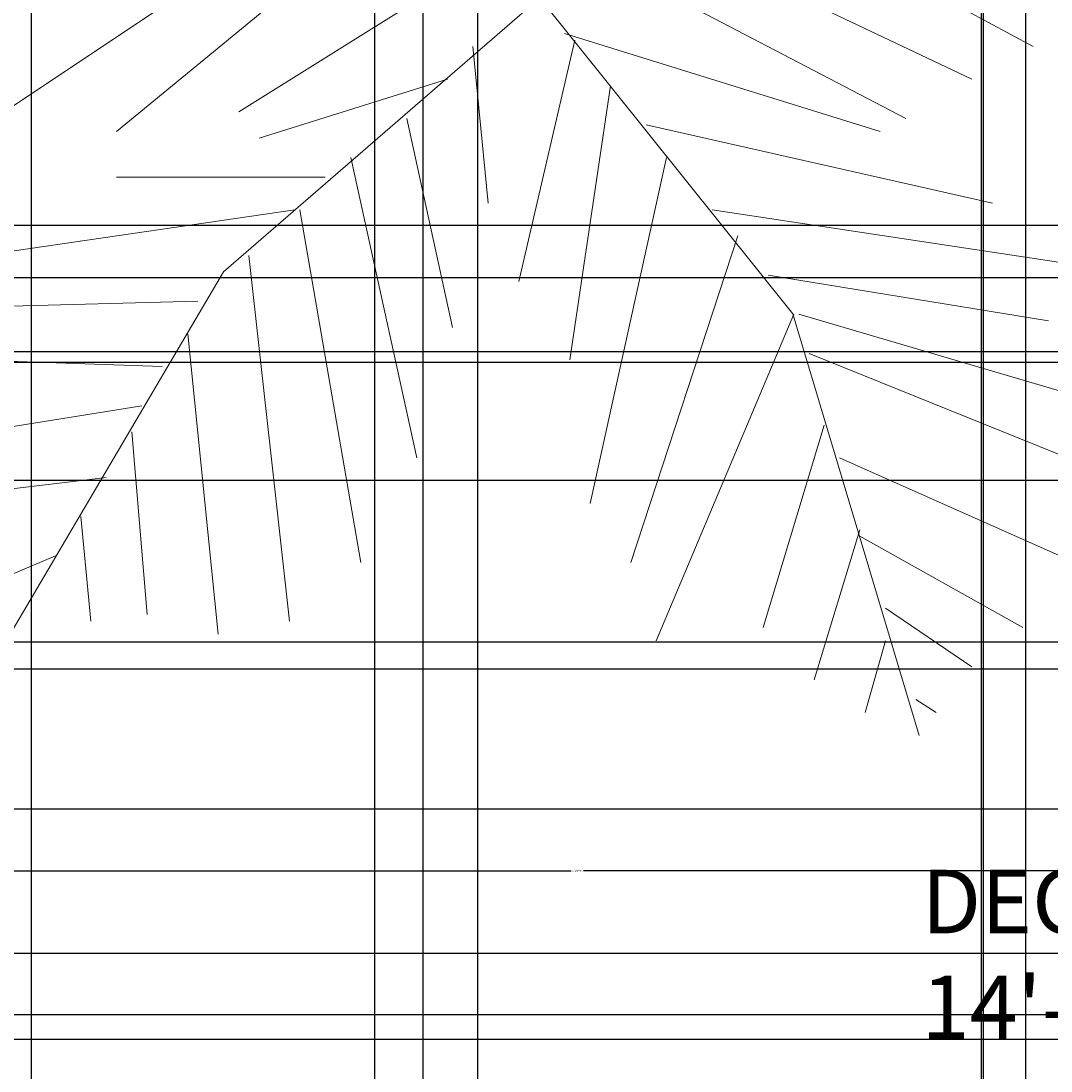
# Model space of a CAD drawing. Units: inches. Extents: x 818 to 1898, y 976 to 2364.
# Tile 62 of 96: x 1083 to 1180, y 1873 to 1972. Entities that reach past the tile are written whole.
import ezdxf

# ---------------------------------------------------------------- set-up
doc = ezdxf.new("R2010")
doc.units = ezdxf.units.IN
doc.header["$LTSCALE"] = 5
doc.header["$MEASUREMENT"] = 0
for name, color, linetype, lineweight in [('A-ANNO-DIMS', 2, 'Continuous', 18), ('A-AREA-IDEN', 7, 'Continuous', 18), ('L-PLNT-BEDS', 94, 'Continuous', 18)]:
    doc.layers.add(name, color=color, linetype=linetype, lineweight=lineweight)
doc.layers.add('L-PLNT', color=116, linetype='Continuous', lineweight=13, true_color=0x136734)
doc.styles.get("Standard").update_dxf_attribs({"font": 'arial.ttf'})
doc.dimstyles.get("Standard").update_dxf_attribs({"dimtxt": 0.18, "dimasz": 0.18, "dimexe": 0.18, "dimexo": 0.0625, "dimgap": 0.09, "dimtad": 0, "dimtih": 1, "dimtoh": 1, "dimdec": 4, "dimzin": 0, "dimdsep": 46, "dimtxsty": 'Standard', "dimcen": 0.09, "dimadec": 0, "dimazin": 0, "dimtfac": 1, "dimtdec": 4, "dimtofl": 0, "dimtmove": 0, "dimatfit": 3, "dimfxl": 1, "dimtolj": 1, "dimtzin": 0, "dimarcsym": 0})

# ---------------------------------------------------------------- blocks, each defined once
blk = doc.blocks.new('PALM-DECK')
for p, q in [((98.208, 77.483), (120.834, 65.14)), ((45.734, 73.779), (23.59, 58.967)), ((89.061, 74.397), (115.057, 62.054)), ((52.955, 72.546), (34.18, 57.116)), ((82.803, 71.928), (108.799, 58.35)), ((65.472, 71.311), (45.734, 58.967)), ((74.194, 69.769), (44.293, 43.854)), ((74.194, 69.769), (98.115, 39.868)), ((77.507, 65.757), (72.213, 42.922)), ((76.545, 66.373), (106.393, 57.116)), ((67.879, 65.14), (69.324, 50.328)), ((65.472, 62.054), (47.659, 56.499)), ((80.877, 61.436), (77.026, 35.515)), ((61.621, 58.35), (65.953, 38.601)), ((84.247, 57.734), (116.983, 50.328)), ((56.325, 54.648), (62.583, 26.258)), ((86.173, 54.648), (78.952, 21.938)), ((53.919, 52.795), (34.18, 52.795)), ((51.03, 49.71), (17.331, 44.773)), ((51.511, 49.71), (57.289, 16.383)), ((90.505, 49.71), (123.241, 44.773)), ((92.912, 47.242), (82.803, 16.383)), ((46.697, 45.389), (50.548, 10.828)), ((44.293, 43.854), (24.359, 9.967)), ((95.801, 43.538), (122.279, 39.218)), ((41.883, 41.069), (17.812, 40.452)), ((98.208, 39.836), (85.21, 8.977)), ((98.115, 39.868), (110.075, 0)), ((98.69, 39.836), (128.056, 31.195)), ((40.92, 37.983), (43.808, 9.593)), ((99.652, 36.132), (125.649, 25.64)), ((38.514, 34.897), (20.701, 35.515)), ((36.587, 31.195), (17.331, 28.109)), ((101.097, 29.344), (95.32, 10.211)), ((35.625, 28.726), (37.069, 11.446)), ((102.541, 26.258), (126.13, 15.766)), ((33.218, 24.406), (17.812, 22.554)), ((30.81, 20.703), (31.773, 10.828)), ((104.467, 19.469), (100.133, 5.273)), ((104.467, 18.852), (119.872, 10.211)), ((28.403, 16.999), (19.737, 13.297)), ((106.874, 12.063), (115.057, 6.508)), ((106.874, 8.977), (104.948, 2.187)), ((109.762, 3.422), (111.687, 2.187))]:
    blk.add_line(p, q)
blk = doc.blocks.new('*D29')
at = {"layer": 'A-ANNO-DIMS', "color": 0, "lineweight": -2, "ltscale": 5, "transparency": 16777216}
for p, q in [((1064.31, 1870.244), (1064.31, 1892.189)), ((1064.49, 1892.009), (1134.729, 1892.009)), ((1206.147, 1892.009), (1135.908, 1892.009)), ((1206.327, 1870.244), (1206.327, 1892.189))]:
    blk.add_line(p, q, dxfattribs=at)
at = {"layer": 'A-ANNO-DIMS', "color": 0, "ltscale": 5, "transparency": 16777216}
for points in [[(1064.49, 1892.039), (1064.49, 1891.979), (1064.31, 1892.009)], [(1206.147, 1892.039), (1206.147, 1891.979), (1206.327, 1892.009)]]:
    blk.add_solid(points, dxfattribs=at)
at = {"layer": 'Defpoints', "color": 0, "ltscale": 5, "transparency": 16777216}
for p in [(1206.327, 1892.009), (1064.31, 1870.181), (1206.327, 1870.181)]:
    blk.add_point(p, dxfattribs=at)
at = {"layer": 'A-ANNO-DIMS', "color": 0, "ltscale": 5, "transparency": 16777216, "insert": (1135.319, 1892.009), "char_height": 0.18, "attachment_point": 5}
blk.add_mtext('\\A1;142 TYP.', dxfattribs=at)
blk = doc.blocks.new('*D59')
at = {"layer": 'A-ANNO-DIMS', "color": 0, "lineweight": -2, "ltscale": 5, "transparency": 16777216}
for p, q in [((1251.643, 2300.393), (818.026, 2300.393)), ((818.206, 2300.213), (818.206, 1669.95)), ((818.206, 1039.323), (818.206, 1669.586)), ((896.051, 1039.143), (818.026, 1039.143))]:
    blk.add_line(p, q, dxfattribs=at)
at = {"layer": 'A-ANNO-DIMS', "color": 0, "ltscale": 5, "transparency": 16777216}
for points in [[(818.176, 2300.213), (818.236, 2300.213), (818.206, 2300.393)], [(818.176, 1039.323), (818.236, 1039.323), (818.206, 1039.143)]]:
    blk.add_solid(points, dxfattribs=at)
at = {"layer": 'Defpoints', "color": 0, "ltscale": 5, "transparency": 16777216}
for p in [(818.206, 2300.393), (1251.706, 2300.393), (896.114, 1039.143)]:
    blk.add_point(p, dxfattribs=at)
at = {"layer": 'A-ANNO-DIMS', "color": 0, "ltscale": 5, "transparency": 16777216, "insert": (818.206, 1669.768), "char_height": 0.18, "attachment_point": 5}
blk.add_mtext('\\A1;1261.2', dxfattribs=at)
blk = doc.blocks.new('*D61')
at = {"layer": 'A-ANNO-DIMS', "color": 0, "lineweight": -2, "ltscale": 5, "transparency": 16777216}
for p, q in [((1071.725, 1203.027), (1071.725, 2363.873)), ((1430.725, 1203.027), (1430.725, 2363.873)), ((1071.905, 2363.693), (1250.936, 2363.693)), ((1430.545, 2363.693), (1251.514, 2363.693))]:
    blk.add_line(p, q, dxfattribs=at)
at = {"layer": 'A-ANNO-DIMS', "color": 0, "ltscale": 5, "transparency": 16777216}
for points in [[(1071.905, 2363.723), (1071.905, 2363.663), (1071.725, 2363.693)], [(1430.545, 2363.723), (1430.545, 2363.663), (1430.725, 2363.693)]]:
    blk.add_solid(points, dxfattribs=at)
at = {"layer": 'Defpoints', "color": 0, "ltscale": 5, "transparency": 16777216}
for p in [(1430.725, 2363.693), (1071.725, 1202.964), (1430.725, 1202.964)]:
    blk.add_point(p, dxfattribs=at)
at = {"layer": 'A-ANNO-DIMS', "color": 0, "ltscale": 5, "transparency": 16777216, "insert": (1251.225, 2363.693), "char_height": 0.18, "attachment_point": 5}
blk.add_mtext('\\A1;359', dxfattribs=at)
blk = doc.blocks.new('*D74')
at = {"layer": 'A-ANNO-DIMS', "color": 0, "lineweight": -2, "ltscale": 5, "transparency": 16777216}
for p, q in [((1590.663, 1940.078), (818.026, 1940.078)), ((818.206, 1939.898), (818.206, 1925.76)), ((818.206, 1911.258), (818.206, 1925.396)), ((1590.663, 1911.078), (818.026, 1911.078))]:
    blk.add_line(p, q, dxfattribs=at)
at = {"layer": 'A-ANNO-DIMS', "color": 0, "ltscale": 5, "transparency": 16777216}
for points in [[(818.176, 1939.898), (818.236, 1939.898), (818.206, 1940.078)], [(818.176, 1911.258), (818.236, 1911.258), (818.206, 1911.078)]]:
    blk.add_solid(points, dxfattribs=at)
at = {"layer": 'Defpoints', "color": 0, "ltscale": 5, "transparency": 16777216}
for p in [(818.206, 1940.078), (1590.725, 1940.078), (1590.725, 1911.078)]:
    blk.add_point(p, dxfattribs=at)
at = {"layer": 'A-ANNO-DIMS', "color": 0, "ltscale": 5, "transparency": 16777216, "insert": (818.206, 1925.578), "char_height": 0.18, "attachment_point": 5}
blk.add_mtext('\\A1;29', dxfattribs=at)
blk = doc.blocks.new('*D82')
at = {"layer": 'A-ANNO-DIMS', "color": 0, "lineweight": -2, "ltscale": 5, "transparency": 16777216}
for p, q in [((1083.725, 1501.141), (1083.725, 2363.873)), ((1197.725, 1501.141), (1197.725, 2363.873)), ((1083.905, 2363.693), (1140.445, 2363.693)), ((1197.545, 2363.693), (1141.005, 2363.693))]:
    blk.add_line(p, q, dxfattribs=at)
at = {"layer": 'A-ANNO-DIMS', "color": 0, "ltscale": 5, "transparency": 16777216}
for points in [[(1083.905, 2363.723), (1083.905, 2363.663), (1083.725, 2363.693)], [(1197.545, 2363.723), (1197.545, 2363.663), (1197.725, 2363.693)]]:
    blk.add_solid(points, dxfattribs=at)
at = {"layer": 'Defpoints', "color": 0, "ltscale": 5, "transparency": 16777216}
for p in [(1197.725, 2363.693), (1083.725, 1501.078), (1197.725, 1501.078)]:
    blk.add_point(p, dxfattribs=at)
at = {"layer": 'A-ANNO-DIMS', "color": 0, "ltscale": 5, "transparency": 16777216, "insert": (1140.725, 2363.693), "char_height": 0.18, "attachment_point": 5}
blk.add_mtext('\\A1;114', dxfattribs=at)
blk = doc.blocks.new('*D93')
at = {"layer": 'A-ANNO-DIMS', "color": 0, "lineweight": -2, "ltscale": 5, "transparency": 16777216}
for p, q in [((1068.338, 1071.118), (1068.338, 2363.873)), ((1120.762, 1071.118), (1120.762, 2363.873)), ((1068.518, 2363.693), (1094.157, 2363.693)), ((1120.582, 2363.693), (1094.942, 2363.693))]:
    blk.add_line(p, q, dxfattribs=at)
at = {"layer": 'A-ANNO-DIMS', "color": 0, "ltscale": 5, "transparency": 16777216}
for points in [[(1068.518, 2363.723), (1068.518, 2363.663), (1068.338, 2363.693)], [(1120.582, 2363.723), (1120.582, 2363.663), (1120.762, 2363.693)]]:
    blk.add_solid(points, dxfattribs=at)
at = {"layer": 'Defpoints', "color": 0, "ltscale": 5, "transparency": 16777216}
for p in [(1120.762, 2363.693), (1068.338, 1071.055), (1120.762, 1071.055)]:
    blk.add_point(p, dxfattribs=at)
at = {"layer": 'A-ANNO-DIMS', "color": 0, "ltscale": 5, "transparency": 16777216, "insert": (1094.55, 2363.693), "char_height": 0.18, "attachment_point": 5}
blk.add_mtext('\\A1;52.42', dxfattribs=at)
blk = doc.blocks.new('*D94')
at = {"layer": 'A-ANNO-DIMS', "color": 0, "lineweight": -2, "ltscale": 5, "transparency": 16777216}
for p, q in [((1120.762, 1071.118), (1120.762, 2363.873)), ((1173.542, 1071.118), (1173.542, 2363.873)), ((1120.942, 2363.693), (1146.758, 2363.693)), ((1173.362, 2363.693), (1147.546, 2363.693))]:
    blk.add_line(p, q, dxfattribs=at)
at = {"layer": 'A-ANNO-DIMS', "color": 0, "ltscale": 5, "transparency": 16777216}
for points in [[(1120.942, 2363.723), (1120.942, 2363.663), (1120.762, 2363.693)], [(1173.362, 2363.723), (1173.362, 2363.663), (1173.542, 2363.693)]]:
    blk.add_solid(points, dxfattribs=at)
at = {"layer": 'Defpoints', "color": 0, "ltscale": 5, "transparency": 16777216}
for p in [(1173.542, 2363.693), (1120.762, 1071.055), (1173.542, 1071.055)]:
    blk.add_point(p, dxfattribs=at)
at = {"layer": 'A-ANNO-DIMS', "color": 0, "ltscale": 5, "transparency": 16777216, "insert": (1147.152, 2363.693), "char_height": 0.18, "attachment_point": 5}
blk.add_mtext('\\A1;52.78', dxfattribs=at)
blk = doc.blocks.new('*D95')
at = {"layer": 'A-ANNO-DIMS', "color": 0, "lineweight": -2, "ltscale": 5, "transparency": 16777216}
for p, q in [((1173.542, 1071.118), (1173.542, 2363.873)), ((1229.647, 1071.118), (1229.647, 2363.873)), ((1173.722, 2363.693), (1201.288, 2363.693)), ((1229.467, 2363.693), (1201.901, 2363.693))]:
    blk.add_line(p, q, dxfattribs=at)
at = {"layer": 'A-ANNO-DIMS', "color": 0, "ltscale": 5, "transparency": 16777216}
for points in [[(1173.722, 2363.723), (1173.722, 2363.663), (1173.542, 2363.693)], [(1229.467, 2363.723), (1229.467, 2363.663), (1229.647, 2363.693)]]:
    blk.add_solid(points, dxfattribs=at)
at = {"layer": 'Defpoints', "color": 0, "ltscale": 5, "transparency": 16777216}
for p in [(1229.647, 2363.693), (1173.542, 1071.055), (1229.647, 1071.055)]:
    blk.add_point(p, dxfattribs=at)
at = {"layer": 'A-ANNO-DIMS', "color": 0, "ltscale": 5, "transparency": 16777216, "insert": (1201.595, 2363.693), "char_height": 0.18, "attachment_point": 5}
blk.add_mtext('\\A1;56.1', dxfattribs=at)
blk = doc.blocks.new('*D109')
at = {"layer": 'A-ANNO-DIMS', "color": 0, "lineweight": -2, "ltscale": 5, "transparency": 16777216}
for p, q in [((1125.917, 1410.117), (1125.917, 2363.873)), ((1203.329, 1409.911), (1203.329, 2363.873)), ((1126.097, 2363.693), (1164.248, 2363.693)), ((1203.149, 2363.693), (1164.999, 2363.693))]:
    blk.add_line(p, q, dxfattribs=at)
at = {"layer": 'A-ANNO-DIMS', "color": 0, "ltscale": 5, "transparency": 16777216}
for points in [[(1126.097, 2363.723), (1126.097, 2363.663), (1125.917, 2363.693)], [(1203.149, 2363.723), (1203.149, 2363.663), (1203.329, 2363.693)]]:
    blk.add_solid(points, dxfattribs=at)
at = {"layer": 'Defpoints', "color": 0, "ltscale": 5, "transparency": 16777216}
for p in [(1203.329, 2363.693), (1125.917, 1410.055), (1203.329, 1409.848)]:
    blk.add_point(p, dxfattribs=at)
at = {"layer": 'A-ANNO-DIMS', "color": 0, "ltscale": 5, "transparency": 16777216, "insert": (1164.623, 2363.693), "char_height": 0.18, "attachment_point": 5}
blk.add_mtext('\\A1;77.41', dxfattribs=at)
blk = doc.blocks.new('*D121')
at = {"layer": 'A-ANNO-DIMS', "color": 0, "lineweight": -2, "ltscale": 5, "transparency": 16777216}
for p, q in [((1766.29, 1884.203), (818.026, 1884.203)), ((818.206, 1884.023), (818.206, 1841.142)), ((818.206, 1797.897), (818.206, 1840.778)), ((1766.29, 1797.717), (818.026, 1797.717))]:
    blk.add_line(p, q, dxfattribs=at)
at = {"layer": 'A-ANNO-DIMS', "color": 0, "ltscale": 5, "transparency": 16777216}
for points in [[(818.176, 1884.023), (818.236, 1884.023), (818.206, 1884.203)], [(818.176, 1797.897), (818.236, 1797.897), (818.206, 1797.717)]]:
    blk.add_solid(points, dxfattribs=at)
at = {"layer": 'Defpoints', "color": 0, "ltscale": 5, "transparency": 16777216}
for p in [(818.206, 1884.203), (1766.352, 1884.203), (1766.352, 1797.717)]:
    blk.add_point(p, dxfattribs=at)
at = {"layer": 'A-ANNO-DIMS', "color": 0, "ltscale": 5, "transparency": 16777216, "insert": (818.206, 1840.96), "char_height": 0.18, "attachment_point": 5}
blk.add_mtext('\\A1;86.49', dxfattribs=at)
blk = doc.blocks.new('*D124')
at = {"layer": 'A-ANNO-DIMS', "color": 0, "lineweight": -2, "ltscale": 5, "transparency": 16777216}
for p, q in [((1131.703, 1974.573), (818.026, 1974.573)), ((818.206, 1974.393), (818.206, 1884.685)), ((818.206, 1794.613), (818.206, 1884.321)), ((1138.442, 1794.433), (818.026, 1794.433))]:
    blk.add_line(p, q, dxfattribs=at)
at = {"layer": 'A-ANNO-DIMS', "color": 0, "ltscale": 5, "transparency": 16777216}
for points in [[(818.176, 1974.393), (818.236, 1974.393), (818.206, 1974.573)], [(818.176, 1794.613), (818.236, 1794.613), (818.206, 1794.433)]]:
    blk.add_solid(points, dxfattribs=at)
at = {"layer": 'Defpoints', "color": 0, "ltscale": 5, "transparency": 16777216}
for p in [(818.206, 1974.573), (1131.765, 1974.573), (1138.504, 1794.433)]:
    blk.add_point(p, dxfattribs=at)
at = {"layer": 'A-ANNO-DIMS', "color": 0, "ltscale": 5, "transparency": 16777216, "insert": (818.206, 1884.503), "char_height": 0.18, "attachment_point": 5}
blk.add_mtext('\\A1;180.14', dxfattribs=at)
blk = doc.blocks.new('*D126')
at = {"layer": 'A-ANNO-DIMS', "color": 0, "lineweight": -2, "ltscale": 5, "transparency": 16777216}
for p, q in [((1035.377, 1252.087), (1035.377, 2363.873)), ((1116.188, 1236.027), (1116.188, 2363.873)), ((1035.557, 2363.693), (1075.406, 2363.693)), ((1116.008, 2363.693), (1076.159, 2363.693))]:
    blk.add_line(p, q, dxfattribs=at)
at = {"layer": 'A-ANNO-DIMS', "color": 0, "ltscale": 5, "transparency": 16777216}
for points in [[(1035.557, 2363.723), (1035.557, 2363.663), (1035.377, 2363.693)], [(1116.008, 2363.723), (1116.008, 2363.663), (1116.188, 2363.693)]]:
    blk.add_solid(points, dxfattribs=at)
at = {"layer": 'Defpoints', "color": 0, "ltscale": 5, "transparency": 16777216}
for p in [(1035.377, 2363.693), (1035.377, 1252.024), (1116.188, 1235.964)]:
    blk.add_point(p, dxfattribs=at)
at = {"layer": 'A-ANNO-DIMS', "color": 0, "ltscale": 5, "transparency": 16777216, "insert": (1075.782, 2363.693), "char_height": 0.18, "attachment_point": 5}
blk.add_mtext('\\A1;80.81', dxfattribs=at)
blk = doc.blocks.new('*D158')
at = {"layer": 'A-ANNO-DIMS', "color": 0, "lineweight": -2, "ltscale": 5, "transparency": 16777216}
for p, q in [((1173.725, 1590.821), (1173.725, 2363.873)), ((1177.725, 1586.821), (1177.725, 2363.873)), ((1173.905, 2363.693), (1175.573, 2363.693)), ((1177.545, 2363.693), (1175.877, 2363.693))]:
    blk.add_line(p, q, dxfattribs=at)
at = {"layer": 'A-ANNO-DIMS', "color": 0, "ltscale": 5, "transparency": 16777216}
for points in [[(1173.905, 2363.723), (1173.905, 2363.663), (1173.725, 2363.693)], [(1177.545, 2363.723), (1177.545, 2363.663), (1177.725, 2363.693)]]:
    blk.add_solid(points, dxfattribs=at)
at = {"layer": 'Defpoints', "color": 0, "ltscale": 5, "transparency": 16777216}
for p in [(1177.725, 2363.693), (1173.725, 1590.758), (1177.725, 1586.758)]:
    blk.add_point(p, dxfattribs=at)
at = {"layer": 'A-ANNO-DIMS', "color": 0, "ltscale": 5, "transparency": 16777216, "insert": (1175.725, 2363.693), "char_height": 0.18, "attachment_point": 5}
blk.add_mtext('\\A1;4', dxfattribs=at)
blk = doc.blocks.new('*D162')
at = {"layer": 'A-ANNO-DIMS', "color": 0, "lineweight": -2, "ltscale": 5, "transparency": 16777216}
for p, q in [((1429.163, 1876.078), (818.026, 1876.078)), ((818.206, 1875.898), (818.206, 1871.76)), ((818.206, 1867.258), (818.206, 1871.396)), ((1429.163, 1867.078), (818.026, 1867.078))]:
    blk.add_line(p, q, dxfattribs=at)
at = {"layer": 'A-ANNO-DIMS', "color": 0, "ltscale": 5, "transparency": 16777216}
for points in [[(818.176, 1875.898), (818.236, 1875.898), (818.206, 1876.078)], [(818.176, 1867.258), (818.236, 1867.258), (818.206, 1867.078)]]:
    blk.add_solid(points, dxfattribs=at)
at = {"layer": 'Defpoints', "color": 0, "ltscale": 5, "transparency": 16777216}
for p in [(1429.225, 1876.078), (818.206, 1867.078), (1429.225, 1867.078)]:
    blk.add_point(p, dxfattribs=at)
at = {"layer": 'A-ANNO-DIMS', "color": 0, "ltscale": 5, "transparency": 16777216, "insert": (818.206, 1871.578), "char_height": 0.18, "attachment_point": 5}
blk.add_mtext('\\A1;9', dxfattribs=at)
blk = doc.blocks.new('*D206')
at = {"layer": 'A-ANNO-DIMS', "color": 0, "lineweight": -2, "ltscale": 5, "transparency": 16777216}
for p, q in [((1590.663, 1911.078), (818.026, 1911.078)), ((818.206, 1910.898), (818.206, 1893.76)), ((818.206, 1876.258), (818.206, 1893.396)), ((1590.663, 1876.078), (818.026, 1876.078))]:
    blk.add_line(p, q, dxfattribs=at)
at = {"layer": 'A-ANNO-DIMS', "color": 0, "ltscale": 5, "transparency": 16777216}
for points in [[(818.176, 1910.898), (818.236, 1910.898), (818.206, 1911.078)], [(818.176, 1876.258), (818.236, 1876.258), (818.206, 1876.078)]]:
    blk.add_solid(points, dxfattribs=at)
at = {"layer": 'Defpoints', "color": 0, "ltscale": 5, "transparency": 16777216}
for p in [(818.206, 1911.078), (1590.725, 1911.078), (1590.725, 1876.078)]:
    blk.add_point(p, dxfattribs=at)
at = {"layer": 'A-ANNO-DIMS', "color": 0, "ltscale": 5, "transparency": 16777216, "insert": (818.206, 1893.578), "char_height": 0.18, "attachment_point": 5}
blk.add_mtext('\\A1;35', dxfattribs=at)
blk = doc.blocks.new('*D211')
at = {"layer": 'A-ANNO-DIMS', "color": 0, "lineweight": -2, "ltscale": 5, "transparency": 16777216}
for p, q in [((1599.66265, 1948.078237), (818.025912, 1948.078237)), ((818.205912, 1947.898237), (818.205912, 1944.758237)), ((818.205912, 1941.258237), (818.205912, 1944.398237)), ((1599.66265, 1941.078237), (818.025912, 1941.078237))]:
    blk.add_line(p, q, dxfattribs=at)
at = {"layer": 'A-ANNO-DIMS', "color": 0, "ltscale": 5, "transparency": 16777216}
for points in [[(818.175912, 1947.898237), (818.235912, 1947.898237), (818.205912, 1948.078237)], [(818.175912, 1941.258237), (818.235912, 1941.258237), (818.205912, 1941.078237)]]:
    blk.add_solid(points, dxfattribs=at)
at = {"layer": 'Defpoints', "color": 0, "ltscale": 5, "transparency": 16777216}
for p in [(818.205912, 1948.078237), (1599.72515, 1948.078237), (1599.72515, 1941.078237)]:
    blk.add_point(p, dxfattribs=at)
at = {"layer": 'A-ANNO-DIMS', "color": 0, "ltscale": 5, "transparency": 16777216, "insert": (818.205912, 1944.578237), "char_height": 0.18, "attachment_point": 5}
blk.add_mtext('\\A1;7', dxfattribs=at)
blk = doc.blocks.new('*D215')
at = {"layer": 'A-ANNO-DIMS', "color": 0, "lineweight": -2, "ltscale": 5, "transparency": 16777216}
for p, q in [((1590.663, 1876.078), (818.026, 1876.078)), ((818.206, 1875.898), (818.206, 1781.76)), ((818.206, 1687.258), (818.206, 1781.396)), ((1511.663, 1687.078), (818.026, 1687.078))]:
    blk.add_line(p, q, dxfattribs=at)
at = {"layer": 'A-ANNO-DIMS', "color": 0, "ltscale": 5, "transparency": 16777216}
for points in [[(818.176, 1875.898), (818.236, 1875.898), (818.206, 1876.078)], [(818.176, 1687.258), (818.236, 1687.258), (818.206, 1687.078)]]:
    blk.add_solid(points, dxfattribs=at)
at = {"layer": 'Defpoints', "color": 0, "ltscale": 5, "transparency": 16777216}
for p in [(818.206, 1876.078), (1590.725, 1876.078), (1511.725, 1687.078)]:
    blk.add_point(p, dxfattribs=at)
at = {"layer": 'A-ANNO-DIMS', "color": 0, "ltscale": 5, "transparency": 16777216, "insert": (818.206, 1781.578), "char_height": 0.18, "attachment_point": 5}
blk.add_mtext('\\A1;189', dxfattribs=at)
blk = doc.blocks.new('*D232')
at = {"layer": 'A-ANNO-DIMS', "color": 0, "lineweight": -2, "ltscale": 5, "transparency": 16777216}
for p, q in [((1303.869, 2008.392), (818.026, 2008.392)), ((818.206, 2008.212), (818.206, 1980.898)), ((818.206, 1953.221), (818.206, 1980.534)), ((1303.869, 1953.041), (818.026, 1953.041))]:
    blk.add_line(p, q, dxfattribs=at)
at = {"layer": 'A-ANNO-DIMS', "color": 0, "ltscale": 5, "transparency": 16777216}
for points in [[(818.176, 2008.212), (818.236, 2008.212), (818.206, 2008.392)], [(818.176, 1953.221), (818.236, 1953.221), (818.206, 1953.041)]]:
    blk.add_solid(points, dxfattribs=at)
at = {"layer": 'Defpoints', "color": 0, "ltscale": 5, "transparency": 16777216}
for p in [(818.206, 2008.392), (1303.931, 2008.392), (1303.931, 1953.041)]:
    blk.add_point(p, dxfattribs=at)
at = {"layer": 'A-ANNO-DIMS', "color": 0, "ltscale": 5, "transparency": 16777216, "insert": (818.206, 1980.716), "char_height": 0.18, "attachment_point": 5}
blk.add_mtext('\\A1;55.35', dxfattribs=at)
blk = doc.blocks.new('*D248')
at = {"layer": 'A-ANNO-DIMS', "color": 0, "lineweight": -2, "ltscale": 5, "transparency": 16777216}
for p, q in [((1258.663, 2019.287), (818.026, 2019.287)), ((818.206, 2019.107), (818.206, 1974.286)), ((818.206, 1929.102), (818.206, 1973.922)), ((1258.663, 1928.922), (818.026, 1928.922))]:
    blk.add_line(p, q, dxfattribs=at)
at = {"layer": 'A-ANNO-DIMS', "color": 0, "ltscale": 5, "transparency": 16777216}
for points in [[(818.176, 2019.107), (818.236, 2019.107), (818.206, 2019.287)], [(818.176, 1929.102), (818.236, 1929.102), (818.206, 1928.922)]]:
    blk.add_solid(points, dxfattribs=at)
at = {"layer": 'Defpoints', "color": 0, "ltscale": 5, "transparency": 16777216}
for p in [(818.206, 2019.287), (1258.725, 2019.287), (1258.725, 1928.922)]:
    blk.add_point(p, dxfattribs=at)
at = {"layer": 'A-ANNO-DIMS', "color": 0, "ltscale": 5, "transparency": 16777216, "insert": (818.206, 1974.104), "char_height": 0.18, "attachment_point": 5}
blk.add_mtext('\\A1;90.37', dxfattribs=at)
blk = doc.blocks.new('*D250')
at = {"layer": 'A-ANNO-DIMS', "color": 0, "lineweight": -2, "ltscale": 5, "transparency": 16777216}
for p, q in [((1250.24, 1913.64), (818.026, 1913.64)), ((818.206, 1913.46), (818.206, 1896.198)), ((818.206, 1878.572), (818.206, 1895.834)), ((1250.24, 1878.392), (818.026, 1878.392))]:
    blk.add_line(p, q, dxfattribs=at)
at = {"layer": 'A-ANNO-DIMS', "color": 0, "ltscale": 5, "transparency": 16777216}
for points in [[(818.176, 1913.46), (818.236, 1913.46), (818.206, 1913.64)], [(818.176, 1878.572), (818.236, 1878.572), (818.206, 1878.392)]]:
    blk.add_solid(points, dxfattribs=at)
at = {"layer": 'Defpoints', "color": 0, "ltscale": 5, "transparency": 16777216}
for p in [(818.206, 1913.64), (1250.303, 1913.64), (1250.303, 1878.392)]:
    blk.add_point(p, dxfattribs=at)
at = {"layer": 'A-ANNO-DIMS', "color": 0, "ltscale": 5, "transparency": 16777216, "insert": (818.206, 1896.016), "char_height": 0.18, "attachment_point": 5}
blk.add_mtext('\\A1;35.25', dxfattribs=at)
blk = doc.blocks.new('*D287')
at = {"layer": 'A-ANNO-DIMS', "color": 0, "lineweight": -2, "ltscale": 5, "transparency": 16777216}
for p, q in [((1303.869, 1953.041), (818.026, 1953.041)), ((818.206, 1952.861), (818.206, 1925.635)), ((818.206, 1898.046), (818.206, 1925.272)), ((1310.963, 1897.866), (818.026, 1897.866))]:
    blk.add_line(p, q, dxfattribs=at)
at = {"layer": 'A-ANNO-DIMS', "color": 0, "ltscale": 5, "transparency": 16777216}
for points in [[(818.176, 1952.861), (818.236, 1952.861), (818.206, 1953.041)], [(818.176, 1898.046), (818.236, 1898.046), (818.206, 1897.866)]]:
    blk.add_solid(points, dxfattribs=at)
at = {"layer": 'Defpoints', "color": 0, "ltscale": 5, "transparency": 16777216}
for p in [(818.206, 1953.041), (1303.931, 1953.041), (1311.025, 1897.866)]:
    blk.add_point(p, dxfattribs=at)
at = {"layer": 'A-ANNO-DIMS', "color": 0, "ltscale": 5, "transparency": 16777216, "insert": (818.206, 1925.454), "char_height": 0.18, "attachment_point": 5}
blk.add_mtext('\\A1;55.17', dxfattribs=at)

msp = doc.modelspace()

# ---------------------------------------------------------------- linework, layer by layer
at = {"layer": 'L-PLNT-BEDS'}
msp.add_line((1083.7251, 2044.0782), (1083.7251, 1211.9642), dxfattribs=at)

# ---------------------------------------------------------------- block references
at = {"layer": 'L-PLNT'}
msp.add_blockref('PALM-DECK', (1057.571, 1904.8049), dxfattribs=at)

# ---------------------------------------------------------------- texts
at = {"layer": 'A-AREA-IDEN', "ltscale": 5, "insert": (1167.8608, 1892.1161), "char_height": 6, "attachment_point": 1}
msp.add_mtext_dynamic_manual_height_columns('DECK\\P14\'-7" X 28\'-8"', width=118.992422, gutter_width=1, heights=[0], dxfattribs=at)

# ---------------------------------------------------------------- dimensions: what is measured, and where the dimension line sits
at = {"layer": 'A-ANNO-DIMS', "ltscale": 5}
for base, p1, p2, override, picture, middle in [((1035.3768, 2363.6929), (1116.1882, 1235.9642), (1035.3768, 1252.0242), {"dimdec": 2, "dimlfac": 1, "dimrnd": 0, "dimzin": 0, "dimdsep": 46, "dimlunit": 2}, '*D126', (1075.7825, 2363.6929)), ((1120.7618, 2363.6929), (1068.3377, 1071.0552), (1120.7618, 1071.0552), {"dimdec": 2, "dimlfac": 1, "dimrnd": 0, "dimzin": 0, "dimdsep": 46, "dimlunit": 2}, '*D93', (1094.5497, 2363.6929)), ((1430.7251, 2363.6929), (1071.7251, 1202.9642), (1430.7251, 1202.9642), {"dimdec": 0, "dimlfac": 1, "dimrnd": 0, "dimzin": 0, "dimdsep": 46, "dimlunit": 2}, '*D61', (1251.2251, 2363.6929)), ((1197.7251, 2363.6929), (1083.7251, 1501.0782), (1197.7251, 1501.0782), {"dimdec": 0, "dimlfac": 1, "dimrnd": 0, "dimzin": 0, "dimdsep": 46, "dimlunit": 2}, '*D82', (1140.7251, 2363.6929)), ((1173.5418, 2363.6929), (1120.7618, 1071.0552), (1173.5418, 1071.0552), {"dimdec": 2, "dimlfac": 1, "dimrnd": 0, "dimzin": 0, "dimdsep": 46, "dimlunit": 2}, '*D94', (1147.1518, 2363.6929)), ((1203.3292, 2363.6929), (1125.9172, 1410.0547), (1203.3292, 1409.8484), {"dimdec": 2, "dimlfac": 1, "dimrnd": 0, "dimzin": 0, "dimdsep": 46, "dimlunit": 2}, '*D109', (1164.6232, 2363.6929)), ((1229.6474, 2363.6929), (1173.5418, 1071.0552), (1229.6474, 1071.0552), {"dimdec": 1, "dimlfac": 1, "dimrnd": 0, "dimzin": 0, "dimdsep": 46, "dimlunit": 2}, '*D95', (1201.5946, 2363.6929)), ((1177.7251, 2363.6929), (1173.7251, 1590.7585), (1177.7251, 1586.7585), {"dimdec": 0, "dimlfac": 1, "dimrnd": 0, "dimzin": 0, "dimdsep": 46, "dimlunit": 2}, '*D158', (1175.7251, 2363.6929))]:
    dim = msp.add_linear_dim(base=base, p1=p1, p2=p2, dimstyle='Standard', override=override, dxfattribs=at)
    dim.commit()
    dim.dimension.update_dxf_attribs({"geometry": picture, "text_midpoint": middle})
for base, p1, p2, override, picture, middle in [((818.2059, 2300.3929), (896.1138, 1039.1433), (1251.7057, 2300.3929), {"dimdec": 1, "dimlfac": 1, "dimrnd": 0, "dimzin": 0, "dimdsep": 46, "dimlunit": 2}, '*D59', (818.2059, 1669.7681)), ((818.2059, 2019.2871), (1258.7251, 1928.9218), (1258.7251, 2019.2871), {"dimdec": 2, "dimlfac": 1, "dimrnd": 0, "dimzin": 0, "dimdsep": 46, "dimlunit": 2}, '*D248', (818.2059, 1974.1044)), ((818.2059, 2008.3917), (1303.9314, 1953.0408), (1303.9314, 2008.3917), {"dimdec": 2, "dimlfac": 1, "dimrnd": 0, "dimzin": 0, "dimdsep": 46, "dimlunit": 2}, '*D232', (818.2059, 1980.7163)), ((818.2059, 1974.5735), (1138.5041, 1794.4325), (1131.7651, 1974.5735), {"dimdec": 2, "dimlfac": 1, "dimrnd": 0, "dimzin": 0, "dimdsep": 46, "dimlunit": 2}, '*D124', (818.2059, 1884.503)), ((818.2059, 1953.0408), (1311.025, 1897.8663), (1303.9314, 1953.0408), {"dimdec": 2, "dimlfac": 1, "dimrnd": 0, "dimzin": 0, "dimdsep": 46, "dimlunit": 2}, '*D287', (818.2059, 1925.4536)), ((818.2059, 1948.0782), (1599.7251, 1941.0782), (1599.7251, 1948.0782), {"dimdec": 0, "dimlfac": 1, "dimrnd": 0, "dimzin": 0, "dimdsep": 46, "dimlunit": 2}, '*D211', (818.2059, 1944.5782)), ((818.2059, 1940.0782), (1590.7251, 1911.0782), (1590.7251, 1940.0782), {"dimdec": 0, "dimlfac": 1, "dimrnd": 0, "dimzin": 0, "dimdsep": 46, "dimlunit": 2}, '*D74', (818.2059, 1925.5782)), ((818.2059, 1913.6401), (1250.3029, 1878.3919), (1250.3029, 1913.6401), {"dimdec": 2, "dimlfac": 1, "dimrnd": 0, "dimzin": 0, "dimdsep": 46, "dimlunit": 2}, '*D250', (818.2059, 1896.016)), ((818.2059, 1911.0782), (1590.7251, 1876.0782), (1590.7251, 1911.0782), {"dimdec": 0, "dimlfac": 1, "dimrnd": 0, "dimzin": 0, "dimdsep": 46, "dimlunit": 2}, '*D206', (818.2059, 1893.5782)), ((818.2059, 1884.2031), (1766.3524, 1797.7165), (1766.3524, 1884.2031), {"dimdec": 2, "dimlfac": 1, "dimrnd": 0, "dimzin": 0, "dimdsep": 46, "dimlunit": 2}, '*D121', (818.2059, 1840.9598)), ((818.2059, 1876.0782), (1511.7251, 1687.0782), (1590.7251, 1876.0782), {"dimdec": 0, "dimlfac": 1, "dimrnd": 0, "dimzin": 0, "dimdsep": 46, "dimlunit": 2}, '*D215', (818.2059, 1781.5782)), ((818.2059, 1867.0782), (1429.2251, 1876.0782), (1429.2251, 1867.0782), {"dimdec": 0, "dimlfac": 1, "dimrnd": 0, "dimzin": 0, "dimdsep": 46, "dimlunit": 2}, '*D162', (818.2059, 1871.5782))]:
    dim = msp.add_linear_dim(base=base, p1=p1, p2=p2, angle=90, dimstyle='Standard', override=override, dxfattribs=at)
    dim.commit()
    dim.dimension.update_dxf_attribs({"geometry": picture, "text_midpoint": middle})
dim = msp.add_linear_dim(base=(1206.3272, 1892.009), p1=(1064.3101, 1870.1814), p2=(1206.3272, 1870.1814), text='<> TYP.', dimstyle='Standard', override={"dimdec": 0, "dimlfac": 1, "dimrnd": 0, "dimzin": 0, "dimdsep": 46, "dimlunit": 2}, dxfattribs=at)
dim.commit()
dim.dimension.update_dxf_attribs({"geometry": '*D29', "text_midpoint": (1135.3187, 1892.009)})

doc.saveas('drawing.dxf')
